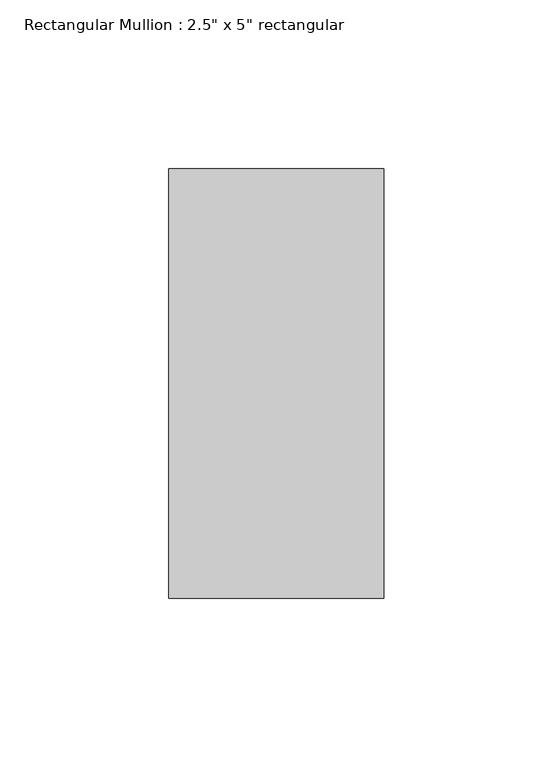
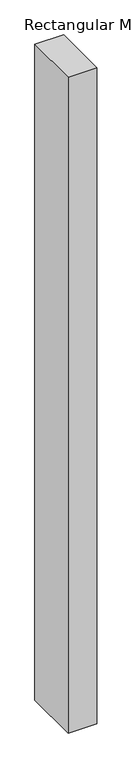
"""IFC4 building model written with IfcOpenShell, lengths in millimetres: member geometry."""

from ifc_helpers import new_model, si_unit, frame, origin, place, context, project, spatial, polyline, outline, extrude, source, transform, mapped, element, save


def member_bb9b20bf(model_context):
    return source(origin(), model_context, "Body", "SweptSolid", [
        extrude(outline(polyline([(31.75, 63.5), (31.75, -63.5), (-31.75, -63.5), (-31.75, 63.5), (31.75, 63.5)])), frame((0.0, 0.0, -1535.0629342), z_axis=(0.0, 0.0, 1.0), x_axis=(1.0, 0.0, 0.0)), (0.0, 0.0, 1.0), 1535.0629342),
    ])


if __name__ == "__main__":
    model = new_model("IFC4")
    model_context = context("Model", 3, world=origin())
    ifc_project = project(units=[si_unit("LENGTHUNIT", "METRE", prefix="MILLI")], contexts=[model_context])
    site = spatial("IfcSite", under=ifc_project)
    building = spatial("IfcBuilding", under=site)
    placement = place(None, origin())
    member_shape = member_bb9b20bf(model_context)
    element("IfcMember", 1, ObjectType="Rectangular Mullion : 2.5\" x 5\" rectangular", at=placement, inside=building, context=model_context, shape_type="MappedRepresentation", body=[
        mapped(member_shape, transform((0.0, 0.0, 0.0), x_axis=(1.0, 0.0, 0.0), y_axis=(0.0, 1.0, 0.0), z_axis=(0.0, 0.0, 1.0))),
    ])
    save(model, "model.ifc")

# Revit data of these elements
# Type "Rectangular Mullion : 2.5\" x 5\" rectangular"
#   built-in parameter 1007304 = 0.416667 (stored number, unit not read)
#   built-in parameter 1007301 = 0.104167 (stored number, unit not read)
#   built-in parameter 1007300 = 0.104167 (stored number, unit not read)
# Element 1 (IfcMember, "Rectangular Mullion : 2.5\" x 5\" rectangular")
#   Materials on its faces: "Aluminum"
# Materials
#   "Aluminum": class "Metal", colour RGB 247 247 247, transparency 0, Description = "Aluminum 6061", Cost = 0
